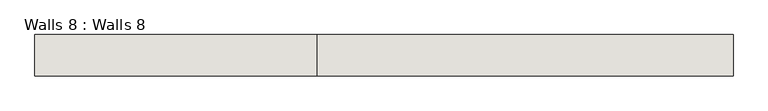
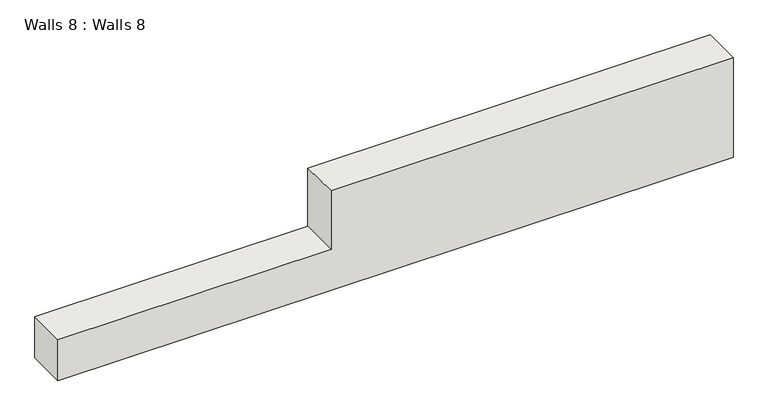
"""IFC4 building model written with IfcOpenShell, lengths in millimetres: wall geometry, Walls 8 : Walls 8."""

from ifc_helpers import new_model, si_unit, frame, origin, place, context, project, spatial, polyline, outline, extrude, source, transform, mapped, element, save


def walls_8_walls_8_6bca06a2(model_context):
    return source(origin(), model_context, "Body", "SweptSolid", [
        extrude(outline(polyline([(3254.9841512, 1204.9616643), (4581.7618503, 1204.9616643), (4581.7618503, -3870.2434506), (3804.3064545, -3870.2434506), (3804.3064545, -7316.7383357), (3254.9841512, -7316.7383357), (3254.9841512, -3870.2434506), (3254.9841512, 1204.9616643)])), frame((0.0, -20435.7210337, 0.0), z_axis=(0.0, 1.0, 0.0), x_axis=(0.0, 0.0, 1.0)), (0.0, 0.0, 1.0), 504.8),
    ])


if __name__ == "__main__":
    model = new_model("IFC4")
    model_context = context("Model", 3, world=origin())
    ifc_project = project(units=[si_unit("LENGTHUNIT", "METRE", prefix="MILLI")], contexts=[model_context])
    site = spatial("IfcSite", under=ifc_project)
    building = spatial("IfcBuilding", under=site)
    placement = place(None, origin())
    walls_8_walls_8_shape = walls_8_walls_8_6bca06a2(model_context)
    element("IfcWall", 1, ObjectType="Walls 8 : Walls 8", at=placement, inside=building, context=model_context, shape_type="MappedRepresentation", body=[
        mapped(walls_8_walls_8_shape, transform((0.0, 0.0, 0.0), x_axis=(1.0, 0.0, 0.0), y_axis=(0.0, 1.0, 0.0), z_axis=(0.0, 0.0, 1.0))),
    ])
    save(model, "model.ifc")

# Revit data of these elements
# Element 1 (IfcWall, "Walls 8 : Walls 8")
#   Materials on its faces: "Default Wall"
# Materials
#   "Default Wall": colour RGB 80 80 80, transparency 0
